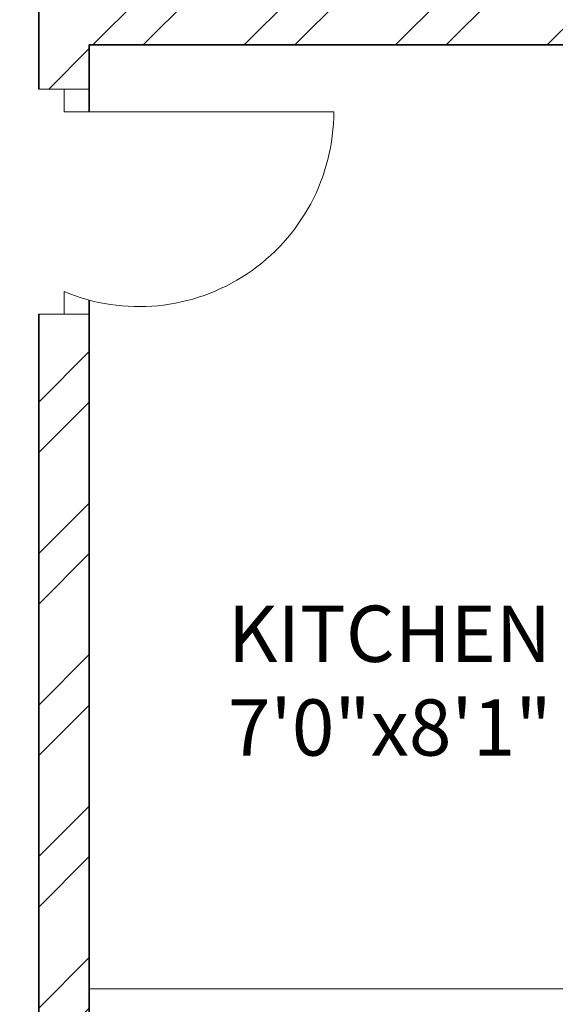
# Model space of a CAD drawing. Units: inches. Extents: x 1885 to 2748, y 783 to 2421.
# Tile 111 of 117: x 2524 to 2571, y 2027 to 2115. Entities that reach past the tile are written whole.
import ezdxf

# ---------------------------------------------------------------- set-up
doc = ezdxf.new("R2010")
doc.units = ezdxf.units.IN
for name, color, linetype, lineweight in [('A-AREA-IDEN', 7, 'Continuous', 18), ('A-DOOR', 31, 'Continuous', 18), ('A-FLOR-CASE', 9, 'Continuous', 18), ('A-WALL', 7, 'Continuous', 35)]:
    doc.layers.add(name, color=color, linetype=linetype, lineweight=lineweight)
doc.layers.add('A-WALL-PATT', color=85, linetype='Continuous', lineweight=13, true_color=0x58ba48)
doc.styles.get("Standard").update_dxf_attribs({"font": 'arial.ttf'})

msp = doc.modelspace()

# ---------------------------------------------------------------- hatches: boundary and pattern name
at = {"layer": 'A-WALL-PATT'}
h = msp.add_hatch(dxfattribs=at)
h.set_pattern_fill('ANSI32', color=256)
h.paths.add_polyline_path([(2007.772, 2318.006), (1980.774, 2318.006), (1980.774, 2281.215), (1985.274, 2281.215), (1985.274, 2313.506), (2007.772, 2313.506), (2007.772, 2315.756)])
h.paths.add_polyline_path([(2094.324, 2318.006), (2067.772, 2318.006), (2067.772, 2313.506), (2094.324, 2313.506), (2094.324, 2315.756)])
h.paths.add_polyline_path([(2131.367, 2315.756), (2131.367, 2318.006), (2131.189, 2318.006), (2112.609, 2318.006), (2112.609, 2313.506), (2117.274, 2313.506), (2117.274, 2255.201), (2121.774, 2255.201), (2121.774, 2313.506), (2131.367, 2313.506)])
h.paths.add_polyline_path([(2190.512, 2318.006), (2155.367, 2318.006), (2155.367, 2313.506), (2169.774, 2313.506), (2169.774, 2229.506), (2121.774, 2229.506), (2121.774, 2233.451), (2119.524, 2233.451), (2117.274, 2233.451), (2117.274, 2201.101), (2121.774, 2201.101), (2121.774, 2225.006), (2169.774, 2225.006), (2169.774, 2165.006), (2306.274, 2165.006), (2306.274, 2066.006), (2310.774, 2066.006), (2344.274, 2066.006), (2486.274, 2066.006), (2486.274, 1886.006), (2483.02, 1886.006), (2483.02, 1881.506), (2486.274, 1881.506), (2486.274, 1880.678), (2490.774, 1880.678), (2490.774, 2070.506), (2344.274, 2070.506), (2310.774, 2070.506), (2310.774, 2165.006), (2310.774, 2173.636), (2308.524, 2173.636), (2306.274, 2173.636), (2306.274, 2169.506), (2174.274, 2169.506), (2174.274, 2313.506), (2190.512, 2313.506), (2190.512, 2315.756)])
h.paths.add_polyline_path([(1985.274, 2221.215), (1980.774, 2221.215), (1980.774, 2165.006), (1992.774, 2165.006), (1992.774, 2141.927), (1997.274, 2141.927), (1997.274, 2165.006), (2117.274, 2165.006), (2117.274, 2163.126), (2121.774, 2163.126), (2121.774, 2172.734), (2119.524, 2172.734), (2117.274, 2172.734), (2117.274, 2169.506), (1985.274, 2169.506)])
h.paths.add_polyline_path([(1997.274, 2105.927), (1992.774, 2105.927), (1992.774, 2070.506), (2016.774, 2070.506), (2016.774, 2059.123), (2019.024, 2059.123), (2021.274, 2059.123), (2021.274, 2070.506), (2117.274, 2070.506), (2117.274, 2022.506), (2114.423, 2022.506), (2114.423, 2018.006), (2123.627, 2018.006), (2123.627, 2020.256), (2123.627, 2022.506), (2121.774, 2022.506), (2121.774, 2142.587), (2119.524, 2142.587), (2117.274, 2142.587), (2117.274, 2075.006), (1997.274, 2075.006)])
h.paths.add_polyline_path([(2092.029, 2020.256), (2092.029, 2022.506), (2021.274, 2022.506), (2021.274, 2035.123), (2016.774, 2035.123), (2016.774, 2018.006), (2016.774, 1978.784), (2021.274, 1978.784), (2021.274, 2018.006), (2092.029, 2018.006)])
h.paths.add_polyline_path([(2260.938, 2022.506), (2153.105, 2022.506), (2153.105, 2020.256), (2153.105, 2018.006), (2155.274, 2018.006), (2155.274, 1886.006), (2107.629, 1886.006), (2107.629, 1881.506), (2182.911, 1881.506), (2182.911, 1883.756), (2182.911, 1886.006), (2159.774, 1886.006), (2159.774, 2018.006), (2260.938, 2018.006), (2260.938, 2020.256)])
h.paths.add_polyline_path([(2047.629, 1883.756), (2047.629, 1886.006), (2021.274, 1886.006), (2021.274, 1918.784), (2019.024, 1918.784), (2016.774, 1918.784), (2016.774, 1881.506), (2047.629, 1881.506)])
h.paths.add_polyline_path([(2306.361, 1883.756), (2306.361, 1886.006), (2296.274, 1886.006), (2296.274, 1982.006), (2316.535, 1982.006), (2316.535, 1984.256), (2316.535, 1986.506), (2296.274, 1986.506), (2296.274, 2022.506), (2289.276, 2022.506), (2289.276, 2018.006), (2291.774, 2018.006), (2291.774, 1886.006), (2242.911, 1886.006), (2242.911, 1881.506), (2306.361, 1881.506)], flags=17)
h.paths.add_polyline_path([(1985.274, 1843.006), (2021.6, 1843.006), (2021.534, 1845.441), (2021.477, 1847.506), (1980.774, 1847.506), (1980.774, 1809.446), (1985.274, 1809.446)])
h.paths.add_polyline_path([(2131.482, 1845.256), (2131.482, 1847.506), (2081.534, 1847.506), (2081.534, 1843.006), (2117.274, 1843.006), (2117.274, 1784.147), (2119.524, 1784.147), (2121.774, 1784.147), (2121.774, 1843.006), (2131.482, 1843.006)])
h.paths.add_polyline_path([(2203.886, 1847.506), (2155.482, 1847.506), (2155.482, 1843.006), (2169.774, 1843.006), (2169.774, 1759.006), (2121.774, 1759.006), (2121.774, 1761.457), (2117.274, 1761.457), (2117.274, 1730.429), (2121.774, 1730.429), (2121.774, 1754.506), (2177.421, 1754.506), (2177.421, 1756.756), (2177.421, 1759.006), (2174.274, 1759.006), (2174.274, 1843.006), (2203.886, 1843.006)])
h.paths.add_polyline_path([(2335.554, 1845.256), (2335.554, 1847.506), (2239.886, 1847.506), (2239.886, 1843.006), (2306.274, 1843.006), (2306.274, 1759.006), (2199.486, 1759.006), (2199.486, 1754.506), (2310.774, 1754.506), (2310.774, 1843.006), (2335.554, 1843.006)])
h.paths.add_polyline_path([(2348.774, 2022.506), (2344.274, 2022.506), (2344.274, 1986.506), (2341.681, 1986.506), (2341.681, 1982.006), (2344.274, 1982.006), (2344.274, 1886.006), (2330.361, 1886.006), (2330.361, 1881.506), (2361.627, 1881.506), (2361.627, 1883.756), (2361.627, 1886.006), (2348.774, 1886.006)], flags=17)
h.paths.add_polyline_path([(2283.251, 2315.756), (2283.251, 2318.006), (2238.512, 2318.006), (2238.512, 2313.506), (2283.251, 2313.506)], flags=17)
h.paths.add_polyline_path([(2363.274, 2348.006), (2388.677, 2348.006), (2388.677, 2350.256), (2388.677, 2352.506), (2358.774, 2352.506), (2358.774, 2348.006), (2358.774, 2318.006), (2344.481, 2318.006), (2344.481, 2313.506), (2358.774, 2313.506), (2358.774, 2229.506), (2310.774, 2229.506), (2310.774, 2231.952), (2306.274, 2231.952), (2306.274, 2205.611), (2310.774, 2205.611), (2310.774, 2225.006), (2358.774, 2225.006), (2358.774, 2211.506), (2452.329, 2211.506), (2452.329, 2213.756), (2452.329, 2216.006), (2363.274, 2216.006), (2363.274, 2318.006)])
h.paths.add_polyline_path([(2310.774, 2313.506), (2320.481, 2313.506), (2320.481, 2315.756), (2320.481, 2318.006), (2302.728, 2318.006), (2302.728, 2313.506), (2306.274, 2313.506), (2306.274, 2251.076), (2310.774, 2251.076)], flags=17)
h.paths.add_polyline_path([(2490.774, 2352.506), (2486.274, 2352.506), (2448.677, 2352.506), (2448.677, 2348.006), (2486.274, 2348.006), (2486.274, 2318.006), (2486.274, 2216.006), (2481.78, 2216.006), (2481.78, 2211.506), (2486.274, 2211.506), (2486.274, 2165.006), (2493.289, 2165.006), (2493.289, 2167.256), (2493.289, 2169.506), (2490.774, 2169.506), (2490.774, 2313.506), (2494.429, 2313.506), (2494.429, 2318.006), (2490.774, 2318.006)])
h.paths.add_polyline_path([(2534.653, 2318.006), (2515.691, 2318.006), (2515.691, 2313.506), (2534.653, 2313.506), (2534.653, 2315.756)])
h.paths.add_polyline_path([(2618.274, 2318.006), (2594.653, 2318.006), (2594.653, 2313.506), (2613.774, 2313.506), (2613.774, 2281.706), (2618.274, 2281.706)])
h.paths.add_polyline_path([(2618.274, 2221.706), (2613.774, 2221.706), (2613.774, 2169.506), (2554.019, 2169.506), (2554.019, 2165.006), (2613.774, 2165.006), (2613.774, 2152.878), (2618.274, 2152.878)])
h.paths.add_polyline_path([(2618.274, 2128.878), (2616.024, 2128.878), (2613.774, 2128.878), (2613.774, 2117.006), (2529.774, 2117.006), (2529.774, 2165.006), (2532.848, 2165.006), (2532.848, 2169.506), (2522.867, 2169.506), (2522.867, 2165.006), (2525.274, 2165.006), (2525.274, 2117.006), (2525.274, 2112.506), (2525.274, 2108.576), (2529.774, 2108.576), (2529.774, 2112.506), (2613.774, 2112.506), (2613.774, 2080.19), (2618.274, 2080.19)])
h.paths.add_polyline_path([(2618.274, 2044.19), (2616.024, 2044.19), (2613.774, 2044.19), (2613.774, 2015.506), (2529.774, 2015.506), (2529.774, 2088.582), (2527.524, 2088.582), (2525.274, 2088.582), (2525.274, 2011.006), (2613.774, 2011.006), (2613.774, 1956.755), (2618.274, 1956.755)])
h.paths.add_polyline_path([(2618.274, 1881.506), (2618.274, 1896.755), (2613.774, 1896.755), (2613.774, 1881.506), (2613.774, 1847.506), (2592.715, 1847.506), (2592.715, 1843.006), (2613.774, 1843.006), (2613.774, 1765.006), (2613.774, 1760.506), (2609.621, 1760.506), (2609.621, 1756.006), (2613.774, 1756.006), (2613.774, 1660.006), (2608.544, 1660.006), (2608.544, 1655.506), (2613.774, 1655.506), (2613.774, 1508.158), (2618.274, 1508.158)])
h.paths.add_polyline_path([(2565.774, 1843.006), (2568.997, 1843.006), (2568.997, 1847.506), (2490.774, 1847.506), (2490.774, 1849.7), (2488.524, 1849.7), (2486.274, 1849.7), (2486.274, 1847.506), (2477.274, 1847.506), (2477.274, 1838.506), (2477.274, 1821.493), (2486.274, 1821.493), (2486.274, 1838.506), (2561.274, 1838.506), (2561.274, 1765.006), (2486.274, 1765.006), (2486.274, 1786.157), (2477.274, 1786.157), (2477.274, 1765.006), (2477.274, 1756.006), (2486.274, 1756.006), (2565.774, 1756.006), (2585.621, 1756.006), (2585.621, 1758.256), (2585.621, 1760.506), (2565.774, 1760.506), (2565.774, 1765.006)])
h.paths.add_polyline_path([(2486.274, 1651.006), (2561.274, 1651.006), (2561.274, 1567.006), (2486.274, 1567.006), (2486.274, 1591.321), (2477.274, 1591.321), (2477.274, 1567.006), (2477.274, 1558.006), (2477.274, 1555.439), (2481.774, 1555.439), (2481.774, 1558.006), (2568.653, 1558.006), (2568.653, 1560.256), (2568.653, 1562.506), (2565.774, 1562.506), (2565.774, 1655.506), (2584.544, 1655.506), (2584.544, 1657.756), (2584.544, 1660.006), (2565.774, 1660.006), (2486.274, 1660.006), (2477.274, 1660.006), (2477.274, 1651.006), (2477.274, 1632.989), (2486.274, 1632.989)])
h.paths.add_polyline_path([(2449.967, 1883.756), (2449.967, 1886.006), (2421.627, 1886.006), (2421.627, 1881.506), (2449.967, 1881.506)], flags=17)
h.paths.add_polyline_path([(2447.274, 1847.506), (2395.554, 1847.506), (2395.554, 1843.006), (2442.774, 1843.006), (2442.774, 1809.27), (2447.274, 1809.27)])
h.paths.add_polyline_path([(1985.274, 1749.446), (1980.774, 1749.446), (1980.774, 1694.504), (1985.274, 1694.504), (1985.274, 1694.506), (1986.897, 1694.506), (1986.897, 1697.78), (1986.897, 1699.006), (1985.274, 1699.006)])
h.paths.add_polyline_path([(2152.774, 1699.006), (2121.774, 1699.006), (2121.774, 1703.668), (2119.524, 1703.668), (2117.274, 1703.668), (2117.274, 1699.006), (2009.219, 1699.006), (2009.219, 1694.506), (2148.274, 1694.506), (2148.274, 1692.631), (2152.774, 1692.631)])
h.paths.add_polyline_path([(2016.274, 1694.506), (2011.774, 1694.506), (2011.774, 1558.006), (2040.806, 1558.006), (2040.806, 1560.256), (2040.806, 1562.506), (2016.274, 1562.506)])
h.paths.add_polyline_path([(2152.774, 1663.017), (2150.524, 1663.017), (2148.274, 1663.017), (2148.274, 1562.506), (2100.806, 1562.506), (2100.806, 1558.006), (2165.119, 1558.006), (2165.119, 1560.256), (2165.119, 1562.506), (2152.774, 1562.506), (2152.774, 1610.506), (2224.774, 1610.506), (2224.774, 1607.99), (2229.274, 1607.99), (2229.274, 1615.006), (2152.774, 1615.006)])
h.paths.add_polyline_path([(2238.613, 1560.256), (2238.613, 1562.506), (2229.274, 1562.506), (2229.274, 1588.756), (2227.024, 1588.763), (2224.774, 1588.771), (2224.774, 1562.506), (2189.119, 1562.506), (2189.119, 1558.006), (2238.613, 1558.006)])
h.paths.add_polyline_path([(2336.024, 1560.256), (2336.024, 1562.506), (2310.774, 1562.506), (2310.774, 1656.347), (2308.524, 1656.347), (2306.274, 1656.347), (2306.274, 1562.506), (2286.613, 1562.506), (2286.613, 1558.006), (2336.024, 1558.006)])
h.paths.add_polyline_path([(2447.274, 1690.968), (2445.024, 1690.968), (2442.774, 1690.968), (2442.774, 1687.006), (2306.274, 1687.006), (2306.274, 1680.75), (2310.774, 1680.75), (2310.774, 1682.506), (2442.774, 1682.506), (2442.774, 1562.506), (2396.024, 1562.506), (2396.024, 1558.006), (2447.274, 1558.006)])
h.paths.add_polyline_path([(2447.274, 1749.27), (2445.024, 1749.27), (2442.774, 1749.27), (2442.774, 1717.232), (2447.274, 1717.232)])
h.paths.add_polyline_path([(2044.674, 1521.756), (2044.674, 1524.006), (2007.274, 1524.006), (2007.274, 1503.49), (2009.524, 1503.49), (2011.774, 1503.49), (2011.774, 1519.506), (2044.674, 1519.506)])
h.paths.add_polyline_path([(2177.969, 1521.756), (2177.969, 1524.006), (2104.674, 1524.006), (2104.674, 1519.506), (2145.774, 1519.506), (2145.774, 1387.506), (2143.37, 1387.506), (2143.37, 1383.006), (2251.585, 1383.006), (2251.585, 1385.256), (2251.585, 1387.506), (2150.274, 1387.506), (2150.274, 1519.506), (2177.969, 1519.506)])
h.paths.add_polyline_path([(2298.704, 1524.006), (2237.969, 1524.006), (2237.969, 1519.506), (2282.274, 1519.506), (2282.274, 1387.506), (2279.683, 1387.506), (2279.683, 1383.006), (2286.774, 1383.006), (2286.774, 1419.006), (2312.451, 1419.006), (2312.451, 1421.256), (2312.451, 1423.506), (2286.774, 1423.506), (2286.774, 1519.506), (2298.704, 1519.506), (2298.704, 1521.722)], flags=17)
h.paths.add_polyline_path([(2361.897, 1521.756), (2361.897, 1524.006), (2322.704, 1524.006), (2322.704, 1519.506), (2334.774, 1519.506), (2334.774, 1423.506), (2331.93, 1423.506), (2331.93, 1419.006), (2334.774, 1419.006), (2334.774, 1387.506), (2334.774, 1383.228), (2339.274, 1383.228), (2339.274, 1387.506), (2339.274, 1519.506), (2361.897, 1519.506)], flags=17)
h.paths.add_polyline_path([(2447.274, 1521.756), (2447.274, 1524.006), (2421.897, 1524.006), (2421.897, 1519.506), (2447.274, 1519.506)], flags=17)
h.paths.add_polyline_path([(2481.774, 1529.6), (2479.524, 1529.6), (2477.274, 1529.6), (2477.274, 1524.006), (2474.489, 1524.006), (2474.489, 1519.506), (2477.274, 1519.506), (2477.274, 1334.506), (2296.774, 1334.506), (2296.774, 1240.506), (2160.274, 1240.506), (2160.274, 1180.506), (2112.274, 1180.506), (2112.274, 1207.692), (2110.024, 1207.692), (2107.774, 1207.692), (2107.774, 1171.609), (2112.274, 1171.609), (2112.274, 1176.006), (2160.274, 1176.006), (2160.274, 1092.006), (2144.221, 1092.006), (2144.221, 1087.506), (2189.497, 1087.506), (2189.497, 1089.756), (2189.497, 1092.006), (2164.774, 1092.006), (2164.774, 1236.006), (2296.774, 1236.006), (2296.774, 1231.912), (2301.274, 1231.912), (2301.274, 1330.006), (2481.774, 1330.006), (2481.774, 1387.506)])
h.paths.add_polyline_path([(2618.274, 1448.158), (2613.774, 1448.158), (2613.774, 1382.506), (2529.774, 1382.506), (2525.274, 1382.506), (2525.274, 1307.062), (2529.774, 1307.062), (2529.774, 1378.006), (2613.774, 1378.006), (2613.774, 1354.988), (2618.274, 1354.988)])
h.paths.add_polyline_path([(2618.274, 1318.988), (2613.774, 1318.988), (2613.774, 1281.006), (2529.774, 1281.006), (2529.774, 1283.786), (2527.524, 1283.786), (2525.274, 1283.786), (2525.274, 1228.506), (2516.794, 1228.506), (2516.794, 1224.006), (2533.484, 1224.006), (2533.484, 1226.256), (2533.484, 1228.506), (2529.774, 1228.506), (2529.774, 1276.506), (2613.774, 1276.506), (2613.774, 1266.02), (2618.274, 1266.02)])
h.paths.add_polyline_path([(2618.274, 1134.964), (2613.774, 1134.964), (2613.774, 1092.006), (2594.545, 1092.006), (2594.545, 1087.506), (2618.274, 1087.506)])
h.paths.add_polyline_path([(2534.545, 1092.006), (2509.765, 1092.006), (2509.765, 1087.506), (2534.545, 1087.506), (2534.545, 1089.756)])
h.paths.add_polyline_path([(2481.274, 1224.006), (2484.117, 1224.006), (2484.117, 1226.256), (2484.117, 1228.506), (2476.774, 1228.506), (2476.774, 1198.506), (2471.61, 1198.506), (2471.61, 1194.006), (2476.774, 1194.006), (2476.774, 1062.006), (2436.894, 1062.006), (2436.894, 1057.506), (2476.774, 1057.506), (2481.274, 1057.506), (2481.274, 1062.006), (2481.274, 1087.506), (2485.354, 1087.506), (2485.354, 1089.756), (2485.354, 1092.006), (2481.274, 1092.006), (2481.274, 1117.506)])
h.paths.add_polyline_path([(2439.898, 1198.506), (2349.274, 1198.506), (2349.274, 1194.006), (2349.274, 1180.506), (2301.274, 1180.506), (2301.274, 1201.896), (2299.024, 1201.896), (2296.774, 1201.896), (2296.774, 1172.335), (2299.024, 1172.335), (2301.274, 1172.335), (2301.274, 1176.006), (2349.274, 1176.006), (2349.274, 1092.006), (2334.452, 1092.006), (2334.452, 1087.506), (2349.274, 1087.506), (2349.274, 1057.506), (2353.774, 1057.506), (2376.894, 1057.506), (2376.894, 1059.756), (2376.894, 1062.006), (2353.774, 1062.006), (2353.774, 1087.506), (2353.774, 1180.506), (2353.774, 1194.006), (2439.898, 1194.006), (2439.898, 1196.256)])
h.paths.add_polyline_path([(2270.596, 1089.756), (2270.596, 1092.006), (2249.497, 1092.006), (2249.497, 1087.506), (2270.596, 1087.506)], flags=17)
h.paths.add_polyline_path([(2310.452, 1092.006), (2301.274, 1092.006), (2301.274, 1153.292), (2296.774, 1153.292), (2296.774, 1092.006), (2293.786, 1092.006), (2293.786, 1087.506), (2310.452, 1087.506), (2310.452, 1089.756)], flags=17)
h.paths.add_polyline_path([(2112.274, 1150.328), (2110.024, 1150.328), (2107.774, 1150.328), (2107.774, 1092.006), (2104.465, 1092.006), (2104.465, 1087.506), (2120.221, 1087.506), (2120.221, 1089.756), (2120.221, 1092.006), (2112.274, 1092.006)])
h.paths.add_polyline_path([(2082.172, 1092.006), (2058.144, 1092.006), (2058.144, 1087.506), (2082.172, 1087.506), (2082.172, 1089.756)])
h.paths.add_polyline_path([(1975.774, 1145.638), (1971.274, 1145.638), (1971.274, 1087.506), (1980.774, 1087.506), (1998.144, 1087.506), (1998.144, 1089.756), (1998.144, 1092.006), (1985.274, 1092.006), (1975.774, 1092.006)])
h.paths.add_polyline_path([(2112.274, 1244.385), (2110.024, 1244.385), (2107.774, 1244.385), (2107.774, 1240.506), (1992.274, 1240.506), (1992.274, 1271.008), (1987.774, 1271.008), (1987.774, 1240.506), (1980.774, 1240.506), (1975.774, 1240.506), (1971.274, 1240.506), (1971.274, 1205.638), (1975.774, 1205.638), (1975.774, 1236.006), (2107.774, 1236.006), (2107.774, 1233.444), (2112.274, 1233.444), (2112.274, 1236.006)])
h.paths.add_polyline_path([(2112.274, 1383.006), (2114.783, 1383.006), (2114.783, 1385.256), (2114.783, 1387.506), (2102.476, 1387.506), (2102.476, 1383.006), (2107.774, 1383.006), (2107.774, 1335.006), (2011.774, 1335.006), (2011.774, 1349.939), (2007.274, 1349.939), (2007.274, 1335.006), (1987.774, 1335.006), (1987.774, 1330.506), (1987.774, 1307.008), (1992.274, 1307.008), (1992.274, 1330.506), (2007.274, 1330.506), (2107.774, 1330.506), (2107.774, 1264.711), (2112.274, 1264.711)])
h.paths.add_polyline_path([(2077.857, 1387.506), (2011.774, 1387.506), (2011.774, 1390.036), (2009.524, 1390.036), (2007.274, 1390.036), (2007.274, 1373.939), (2011.774, 1373.939), (2011.774, 1383.006), (2077.857, 1383.006)])
h.paths.add_polyline_path([(2011.774, 1443.49), (2007.274, 1443.49), (2007.274, 1410.248), (2011.774, 1410.248)])

# ---------------------------------------------------------------- linework, layer by layer
at = {"layer": 'A-DOOR'}
for p, q in [((2525.274, 2108.576), (2529.774, 2108.576)), ((2529.774, 2108.576), (2527.524, 2108.576)), ((2527.524, 2108.576), (2527.524, 2106.576)), ((2527.524, 2106.576), (2551.524, 2106.576)), ((2527.524, 2088.582), (2527.524, 2090.582)), ((2525.274, 2088.582), (2529.774, 2088.582)), ((2529.774, 2088.582), (2527.524, 2088.582))]:
    msp.add_line(p, q, dxfattribs=at)
msp.add_arc((2534.194, 2106.576), 17.33, 247.36206, 360, dxfattribs=at)
at = {"layer": 'A-FLOR-CASE'}
msp.add_line((2600.531, 2028.584), (2529.774, 2028.584), dxfattribs=at)
at = {"layer": 'A-WALL'}
for p, q in [((2525.274, 2117.006), (2525.274, 2112.506)), ((2525.274, 2112.506), (2525.274, 2108.576)), ((2529.774, 2112.506), (2613.774, 2112.506)), ((2529.774, 2112.506), (2529.774, 2106.576)), ((2529.774, 2089.82), (2529.774, 2015.506)), ((2525.274, 2088.582), (2525.274, 2011.006))]:
    msp.add_line(p, q, dxfattribs=at)

# ---------------------------------------------------------------- texts
at = {"layer": 'A-AREA-IDEN', "insert": (2542.108, 2062.656), "char_height": 5, "attachment_point": 1}
msp.add_mtext_dynamic_manual_height_columns('KITCHEN\\P7\'0"x8\'1"', width=161.34475, gutter_width=12.5, heights=[0], dxfattribs=at)

doc.saveas('drawing.dxf')
